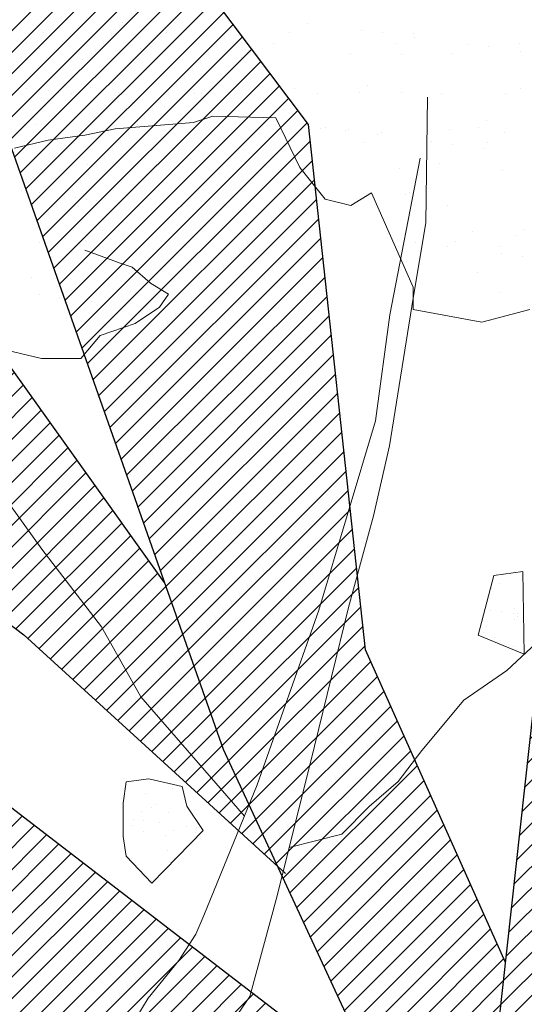
# Model space of a CAD drawing. Units: inches. Extents: x 1986 to 21484, y -1816 to 2016.
# Tile 24 of 85: x 2166.915 to 2172.013, y 1888.377 to 1898.331. Entities that reach past the tile are written whole.
import ezdxf

# ---------------------------------------------------------------- set-up
doc = ezdxf.new("R2010")
doc.units = ezdxf.units.IN
doc.layers.add('L-PLNT', color=84, linetype='Continuous', lineweight=13)
doc.layers.add('vfolhas', color=114, linetype='Continuous', lineweight=5)
doc.layers.add('vfolha2', color=110, linetype='Continuous')
doc.layers.add('vfolhas2', color=102, linetype='Continuous')
pattern_1 = [(45, (-2446.5133113, 50.986076), (-0.004419417382, 0.004419417382), [])]

# ---------------------------------------------------------------- blocks, each defined once
blk = doc.blocks.new('arbusto_PB_verde_grande')
at = {"layer": 'vfolha2'}
h = blk.add_hatch(dxfattribs=at)
h.set_pattern_fill('ANSI31', color=256, scale=0.05, style=0)
h.set_pattern_definition(pattern_1)
h.paths.add_polyline_path([(0.02944, 0.35651), (0.00028, 0.09048), (0.02625, -0.03934), (0.047, 0.06233), (0.06189, 0.09731), (0.09372, 0.26573), (0.09955, 0.43473), (0.08789, 0.61313), (0.0645, 0.72266), (0.04988, 0.6851), (0.0236, 0.51294)])
h.paths.add_polyline_path([(0.30106, 0.43789), (0.14225, 0.24871), (0.26685, 0.30022)])
h.paths.add_polyline_path([(0.37995, 0.22817), (0.23697, 0.15193), (0.18428, 0.09364), (0.11122, 0.04358), (0.02625, -0.03934), (0.28061, 0.04667), (0.36829, 0.07798), (0.46756, 0.11239), (0.61068, 0.19376), (0.71585, 0.27823), (0.55813, 0.25948)])
h.paths.add_polyline_path([(0.56101, -0.29441), (0.72752, -0.32573), (0.59024, -0.2412), (0.42962, -0.15982), (0.02625, -0.03934), (0.14922, -0.14107), (0.18838, -0.16604), (0.41501, -0.24435)])
h.paths.add_polyline_path([(-0.27429, -0.44776), (-0.30352, -0.72628), (-0.23923, -0.64175), (-0.15457, -0.45716), (0.02625, -0.03934), (-0.16328, -0.25376)])
h.paths.add_polyline_path([(-0.51963, -0.24744), (-0.67736, -0.32573), (-0.59558, -0.35072), (-0.40574, -0.32882), (-0.21007, -0.20995), (0.02625, -0.03934), (-0.14874, -0.06595), (-0.31518, -0.09101), (-0.41452, -0.15048)])
h.paths.add_polyline_path([(-0.52546, 0.25007), (-0.70947, 0.24698), (-0.51963, 0.1093), (-0.32979, 0.02167), (-0.07567, -0.0128), (-0.04234, -0.02148), (-0.35024, 0.1312)])
h = blk.add_hatch(dxfattribs=at)
h.set_pattern_fill('ANSI31', color=256, scale=0.05, style=0)
h.set_pattern_definition(pattern_1)
h.paths.add_polyline_path([(-0.18963, 0.29704), (-0.08553, 0.20192), (-0.10785, 0.25007), (-0.13202, 0.31865), (-0.25096, 0.48479), (-0.44952, 0.5505), (-0.37946, 0.43789)])
h.paths.add_polyline_path([(0.07911, -0.4071), (0.08214, -0.50631), (0.17255, -0.6355), (0.18428, -0.44151), (0.14904, -0.29177), (0.02625, -0.03934), (0.03527, -0.25376)])
at = {"layer": 'vfolhas'}
h = blk.add_hatch(dxfattribs=at)
h.set_pattern_fill('ANSI31', color=256, scale=0.05, style=0)
h.set_pattern_definition(pattern_1)
h.paths.add_polyline_path([(-0.07279, 0.50669), (-0.18085, 0.65063), (-0.2334, 0.67253), (-0.20712, 0.53176), (-0.10785, 0.25007), (0.02625, -0.03934), (0.00028, 0.09048), (0.00816, 0.16241), (-0.04939, 0.29079)])
h.paths.add_polyline_path([(0.09902, 0.41929), (0.09372, 0.26573), (0.07906, 0.18814), (0.15506, 0.36901), (0.26606, 0.5505), (0.28356, 0.63504), (0.2485, 0.68819), (0.25145, 0.63504), (0.20178, 0.54426)])
h.paths.add_polyline_path([(0.12295, 0.24073), (0.047, 0.06233), (0.02625, -0.03934), (0.11122, 0.04358), (0.18428, 0.09364), (0.27478, 0.19376), (0.3215, 0.25323), (0.44129, 0.38467), (0.47634, 0.57866), (0.41789, 0.45347), (0.28939, 0.30954)])
h.paths.add_polyline_path([(0.58145, -0.03779), (0.70707, 0.01536), (0.78591, 0.04667), (0.74796, 0.06549), (0.62818, 0.08423), (0.52595, 0.09048), (0.39745, 0.04358), (0.02625, -0.03934), (0.25728, -0.03154), (0.43834, -0.0347)])
h.paths.add_polyline_path([(0.52022, -0.03647), (0.43834, -0.0347), (0.25728, -0.03154), (0.02625, -0.03934), (0.17964, -0.08515), (0.53768, -0.13167), (0.69541, -0.15357), (0.78591, -0.07852), (0.70413, -0.10042)])
h.paths.add_polyline_path([(0.27189, -0.21929), (0.14922, -0.14107), (0.02625, -0.03934), (0.15794, -0.31007), (0.29522, -0.42585), (0.41789, -0.49157), (0.56396, -0.56669), (0.5114, -0.48532), (0.39456, -0.34139)])
h.paths.add_polyline_path([(-0.05818, -0.47591), (-0.02312, -0.61984), (0.047, -0.80134), (0.08494, -0.59794), (0.07911, -0.4071), (0.03527, -0.25376), (0.02625, -0.03934), (-0.03773, -0.26001)])
h.paths.add_polyline_path([(-0.24218, 0.14054), (-0.11073, 0.06858), (0.02625, -0.03934), (-0.04235, 0.10871), (-0.21007, 0.23757), (-0.36485, 0.33145), (-0.47874, 0.40341), (-0.54303, 0.46288), (-0.49041, 0.33145), (-0.39408, 0.22192)])
at = {"layer": 'vfolha2'}
for p, q in [((-0.13202, 0.31865), (-0.25096, 0.48479)), ((-0.37946, 0.43789), (-0.18963, 0.29704)), ((0.00028, 0.09048), (0.02944, 0.35651)), ((-0.18963, 0.29704), (-0.0822, 0.19888))]:
    blk.add_line(p, q, dxfattribs=at)
at = {"layer": 'vfolhas2'}
for p, q in [((-0.07279, 0.50669), (-0.18085, 0.65063)), ((-0.20712, 0.53176), (-0.10785, 0.25007)), ((-0.04939, 0.29079), (-0.07279, 0.50669)), ((0.00816, 0.16241), (-0.04939, 0.29079)), ((-0.10785, 0.25007), (0.02625, -0.03934)), ((-0.04235, 0.10871), (-0.21007, 0.23757))]:
    blk.add_line(p, q, dxfattribs=at)
blk = doc.blocks.new('PLANT-SHRUB')
for p, q in [((2167.9501, 1898.2978), (2167.9501, 1898.2978)), ((2169.8264, 1898.296), (2169.8264, 1898.296)), ((2167.1549, 1898.2015), (2167.1549, 1898.2015)), ((2168.3995, 1898.1993), (2168.3995, 1898.1993)), ((2169.6442, 1898.197), (2169.6442, 1898.197)), ((2170.3692, 1898.2246), (2170.3692, 1898.2246)), ((2170.5773, 1898.1972), (2170.5773, 1898.1972)), ((2170.8888, 1898.1947), (2170.8888, 1898.1947)), ((2170.9022, 1898.1544), (2170.9022, 1898.1544)), ((2166.9864, 1898.0942), (2166.9864, 1898.0942)), ((2167.1119, 1898.0364), (2167.1119, 1898.0364)), ((2168.1343, 1898.0413), (2168.1343, 1898.0413)), ((2168.231, 1898.0919), (2168.231, 1898.0919)), ((2169.4756, 1898.0896), (2169.4756, 1898.0896)), ((2170.7203, 1898.0874), (2170.7203, 1898.0874)), ((2171.445, 1898.0829), (2171.445, 1898.0829)), ((2171.6531, 1898.0555), (2171.6531, 1898.0555)), ((2171.9649, 1898.0851), (2171.9649, 1898.0851)), ((2167.5523, 1897.9333), (2167.5523, 1897.9333)), ((2169.1516, 1897.9471), (2169.1516, 1897.9471)), ((2169.2137, 1898.0024), (2169.2137, 1898.0024)), ((2169.2252, 1898.0146), (2169.2252, 1898.0146)), ((2170.2599, 1897.9891), (2170.2599, 1897.9891)), ((2170.7744, 1897.9824), (2170.7744, 1897.9824)), ((2171.2823, 1897.994), (2171.2823, 1897.994)), ((2171.978, 1898.0128), (2171.978, 1898.0128)), ((2166.9813, 1897.6358), (2166.9813, 1897.6358)), ((2167.6271, 1897.641), (2167.6271, 1897.641)), ((2169.6957, 1897.6326), (2169.6957, 1897.6326)), ((2170.4267, 1897.6638), (2170.4267, 1897.6638)), ((2171.9759, 1897.6316), (2171.9759, 1897.6316)), ((2167.1309, 1897.5472), (2167.1309, 1897.5472)), ((2167.2046, 1897.6147), (2167.2046, 1897.6147)), ((2167.3062, 1897.593), (2167.3062, 1897.593)), ((2167.4389, 1897.5872), (2167.4389, 1897.5872)), ((2168.6733, 1897.6277), (2168.6733, 1897.6277)), ((2168.6835, 1897.585), (2168.6835, 1897.585)), ((2168.7538, 1897.5825), (2168.7538, 1897.5825)), ((2169.9281, 1897.5827), (2169.9281, 1897.5827)), ((2170.353, 1897.5963), (2170.353, 1897.5963)), ((2170.7752, 1897.5937), (2170.7752, 1897.5937)), ((2171.0333, 1897.5479), (2171.0183, 1896.2787)), ((2171.1728, 1897.5805), (2171.1728, 1897.5805)), ((2171.8213, 1897.5804), (2171.8213, 1897.5804)), ((2167.8491, 1897.5215), (2167.8491, 1897.5215)), ((2168.0571, 1897.4942), (2168.0571, 1897.4942)), ((2168.382, 1897.4514), (2168.382, 1897.4514)), ((2168.8651, 1897.3558), (2168.6714, 1897.2912)), ((2169.5017, 1897.3383), (2168.8651, 1897.3558)), ((2169.7439, 1896.8381), (2169.5017, 1897.3383)), ((2167.0867, 1897.2663), (2167.0867, 1897.2663)), ((2168.6714, 1897.2912), (2167.8802, 1897.2267)), ((2168.1091, 1897.2712), (2168.1091, 1897.2712)), ((2170.0007, 1897.2383), (2170.0007, 1897.2383)), ((2171.5545, 1897.2455), (2171.5545, 1897.2455)), ((2171.6282, 1897.313), (2171.6282, 1897.313)), ((2167.5734, 1897.1622), (2167.202, 1897.1138)), ((2167.8802, 1897.2267), (2167.5734, 1897.1622)), ((2169.9552, 1897.2318), (2169.9552, 1897.2318)), ((2170.2088, 1897.2109), (2170.2088, 1897.2109)), ((2170.2347, 1897.219), (2170.2347, 1897.219)), ((2170.5337, 1897.1681), (2170.5337, 1897.1681)), ((2170.566, 1897.1939), (2170.566, 1897.1939)), ((2171.2571, 1897.2239), (2171.2571, 1897.2239)), ((2171.8106, 1897.1917), (2171.8106, 1897.1917)), ((2167.202, 1897.1138), (2166.8629, 1897.0331)), ((2170.3975, 1897.0866), (2170.3975, 1897.0866)), ((2171.0765, 1897.0966), (2171.0765, 1897.0966)), ((2171.2846, 1897.0692), (2171.2846, 1897.0692)), ((2171.6421, 1897.0843), (2171.6421, 1897.0843)), ((2171.6095, 1897.0265), (2171.6095, 1897.0265)), ((2167.602, 1896.8709), (2167.602, 1896.8709)), ((2170.0023, 1896.5154), (2169.7439, 1896.8381)), ((2170.6548, 1895.3462), (2170.9596, 1896.9325)), ((2171.1567, 1896.881), (2171.1567, 1896.881)), ((2170.75, 1896.8236), (2170.75, 1896.8236)), ((2171.7962, 1896.8103), (2171.7962, 1896.8103)), ((2166.9377, 1896.6067), (2166.9377, 1896.6067)), ((2167.1161, 1896.5864), (2167.1161, 1896.5864)), ((2170.4705, 1896.58), (2170.2606, 1896.4509)), ((2170.8904, 1895.628), (2170.4705, 1896.58)), ((2170.809, 1896.5624), (2170.809, 1896.5624)), ((2170.85, 1896.5796), (2170.85, 1896.5796)), ((2167.0615, 1896.4962), (2167.0615, 1896.4962)), ((2167.4806, 1896.5352), (2167.4806, 1896.5352)), ((2167.5132, 1896.4458), (2167.5132, 1896.4458)), ((2167.5869, 1896.5133), (2167.5869, 1896.5133)), ((2167.6886, 1896.5079), (2167.6886, 1896.5079)), ((2170.2606, 1896.4509), (2170.0023, 1896.5154)), ((2171.232, 1896.4538), (2171.232, 1896.4538)), ((2171.0183, 1896.2787), (2170.8904, 1895.5151)), ((2167.754, 1896.1976), (2167.754, 1896.1976)), ((2171.4879, 1896.1908), (2171.4879, 1896.1908)), ((2171.9368, 1896.1441), (2171.9368, 1896.1441)), ((2172.0105, 1896.2116), (2172.0105, 1896.2116)), ((2167.1154, 1896.0813), (2167.1154, 1896.0813)), ((2167.5768, 1896.1008), (2167.5768, 1896.1008)), ((2167.5854, 1896.0903), (2167.5854, 1896.0903)), ((2170.9161, 1896.083), (2170.9161, 1896.083)), ((2171.241, 1896.0402), (2171.241, 1896.0402)), ((2171.3193, 1896.0835), (2171.3193, 1896.0835)), ((2171.771, 1896.0402), (2171.771, 1896.0402)), ((2167.9305, 1895.8701), (2167.5745, 1896.0023)), ((2171.7839, 1895.9687), (2171.7839, 1895.9687)), ((2171.9919, 1895.9413), (2171.9919, 1895.9413)), ((2168.0525, 1895.8295), (2167.9305, 1895.8701)), ((2168.2356, 1895.6669), (2168.0525, 1895.8295)), ((2171.539, 1895.7796), (2171.539, 1895.7796)), ((2167.0363, 1895.7261), (2167.0363, 1895.7261)), ((2168.0587, 1895.731), (2168.0587, 1895.731)), ((2168.4187, 1895.5551), (2168.2356, 1895.6669)), ((2167.1121, 1895.549), (2167.1121, 1895.549)), ((2168.0379, 1895.5833), (2168.0379, 1895.5833)), ((2168.3272, 1895.4229), (2168.4187, 1895.5551)), ((2168.4187, 1895.5551), (2168.4187, 1895.5551)), ((2170.8904, 1895.4022), (2170.8904, 1895.628)), ((2171.7718, 1895.5766), (2171.7718, 1895.5766)), ((2167.3201, 1895.5216), (2167.3201, 1895.5216)), ((2167.645, 1895.4788), (2167.645, 1895.4788)), ((2170.8904, 1895.5151), (2170.6507, 1894.022)), ((2168.083, 1895.2603), (2168.3272, 1895.4229)), ((2170.5087, 1894.2757), (2170.6548, 1895.3462)), ((2171.5847, 1895.2731), (2170.8904, 1895.4022)), ((2172.0691, 1895.4022), (2171.5847, 1895.2731)), ((2167.727, 1895.1384), (2168.083, 1895.2603)), ((2171.5847, 1895.2731), (2171.5847, 1895.2731)), ((2166.4251, 1895.0774), (2167.1371, 1894.9046)), ((2167.5338, 1894.9046), (2167.727, 1895.1384)), ((2167.1371, 1894.9046), (2167.5338, 1894.9046)), ((2169.9359, 1892.3623), (2170.5087, 1894.2757)), ((2167.1381, 1892.979), (2166.4276, 1893.9579)), ((2170.6507, 1894.022), (2170.4886, 1893.314)), ((2170.4886, 1893.314), (2170.2384, 1892.3871)), ((2167.741, 1892.1938), (2167.1381, 1892.979)), ((2171.5456, 1892.1099), (2171.7066, 1892.7104)), ((2171.7066, 1892.7104), (2171.9964, 1892.7533)), ((2171.9964, 1892.7533), (2172.0126, 1891.9166)), ((2171.68, 1892.5784), (2171.68, 1892.5784)), ((2171.7643, 1892.632), (2171.7643, 1892.632)), ((2169.3141, 1890.5948), (2169.9359, 1892.3623)), ((2170.2384, 1892.3871), (2169.8926, 1890.9859)), ((2171.674, 1892.3613), (2171.674, 1892.3613)), ((2171.8369, 1891.7521), (2172.5398, 1892.4105)), ((2171.9153, 1892.377), (2171.9153, 1892.377)), ((2171.778, 1892.3477), (2171.778, 1892.3477)), ((2171.9062, 1892.3249), (2171.9062, 1892.3249)), ((2171.9095, 1892.2646), (2171.9095, 1892.2646)), ((2171.9405, 1892.3263), (2171.9405, 1892.3263)), ((2171.9464, 1892.2983), (2171.9464, 1892.2983)), ((2168.1393, 1891.4839), (2167.741, 1892.1938)), ((2171.6332, 1892.1988), (2171.6332, 1892.1988)), ((2171.5456, 1892.1099), (2171.5456, 1892.1099)), ((2172.0126, 1891.9166), (2171.5456, 1892.1099)), ((2171.6029, 1892.1316), (2171.6029, 1892.1316)), ((2171.7106, 1892.0823), (2171.7106, 1892.0823)), ((2171.9027, 1891.992), (2171.9027, 1891.992)), ((2172.0126, 1891.9166), (2172.0126, 1891.9166)), ((2171.4019, 1891.4502), (2171.8369, 1891.7521)), ((2169.1846, 1890.2781), (2168.1393, 1891.4839)), ((2170.979, 1890.9431), (2171.4019, 1891.4502)), ((2169.8926, 1890.9859), (2169.5176, 1889.4739)), ((2170.7374, 1890.6292), (2170.979, 1890.9431)), ((2167.9597, 1890.4105), (2167.9903, 1890.6245)), ((2167.9903, 1890.6245), (2168.2197, 1890.655)), ((2168.2197, 1890.655), (2168.5562, 1890.5786)), ((2168.5562, 1890.5786), (2168.6021, 1890.38)), ((2168.7741, 1889.2745), (2169.3141, 1890.5948)), ((2170.4473, 1890.3756), (2170.7374, 1890.6292)), ((2168.1813, 1890.5058), (2168.1813, 1890.5058)), ((2168.4612, 1890.5565), (2168.4612, 1890.5565)), ((2167.9597, 1890.0743), (2167.9597, 1890.4105)), ((2168.2874, 1890.3972), (2168.2874, 1890.3972)), ((2168.6021, 1890.38), (2168.7703, 1890.1355)), ((2168.6021, 1890.38), (2168.6021, 1890.38)), ((2170.1694, 1890.0979), (2170.4473, 1890.3756)), ((2168.1491, 1890.3289), (2168.1491, 1890.3289)), ((2168.2505, 1890.3634), (2168.2505, 1890.3634)), ((2168.4222, 1890.3209), (2168.4222, 1890.3209)), ((2168.0516, 1890.1812), (2168.0516, 1890.1812)), ((2168.0632, 1890.2497), (2168.0632, 1890.2497)), ((2168.1672, 1890.236), (2168.1672, 1890.236)), ((2168.3297, 1890.2146), (2168.3297, 1890.2146)), ((2168.6011, 1890.1789), (2168.6011, 1890.1789)), ((2167.9903, 1889.8757), (2167.9597, 1890.0743)), ((2168.1687, 1890.1208), (2168.1687, 1890.1208)), ((2168.7703, 1890.1355), (2168.2503, 1889.6006)), ((2168.3838, 1890.0808), (2168.3838, 1890.0808)), ((2168.468, 1890.1345), (2168.468, 1890.1345)), ((2168.6918, 1890.1141), (2168.6918, 1890.1141)), ((2168.7051, 1890.1652), (2168.7051, 1890.1652)), ((2169.6386, 1889.9619), (2170.1694, 1890.0979)), ((2168.2503, 1889.6006), (2167.9903, 1889.8757)), ((2168.4097, 1889.9359), (2168.4097, 1889.9359)), ((2169.6386, 1889.9619), (2169.6386, 1889.9619)), ((2168.4417, 1889.8127), (2168.4417, 1889.8127)), ((2168.4785, 1889.8465), (2168.4785, 1889.8465)), ((2168.1454, 1889.7215), (2168.1454, 1889.7215)), ((2168.1561, 1889.7357), (2168.1561, 1889.7357)), ((2168.2428, 1889.6305), (2168.2428, 1889.6305)), ((2169.5176, 1889.4739), (2169.239, 1888.4566)), ((2168.6938, 1889.0872), (2168.7741, 1889.2745)), ((2168.5212, 1888.8196), (2168.6938, 1889.0872)), ((2168.2144, 1888.4387), (2168.5212, 1888.8196)), ((2167.9401, 1887.9934), (2168.2144, 1888.4387)), ((2169.239, 1888.4566), (2168.8164, 1887.8423))]:
    blk.add_line(p, q)

msp = doc.modelspace()

# ---------------------------------------------------------------- block references
at = {"layer": 'L-PLNT'}
msp.add_blockref('PLANT-SHRUB', (0, 0), dxfattribs=at)
at = {"layer": 'L-PLNT', "xscale": 24.60366729364114, "yscale": 24.60366729364114, "zscale": 24.60366729364114}
msp.add_blockref('arbusto_PB_verde_grande', (2171.6234, 1884.8051), dxfattribs=at)

doc.saveas('drawing.dxf')
